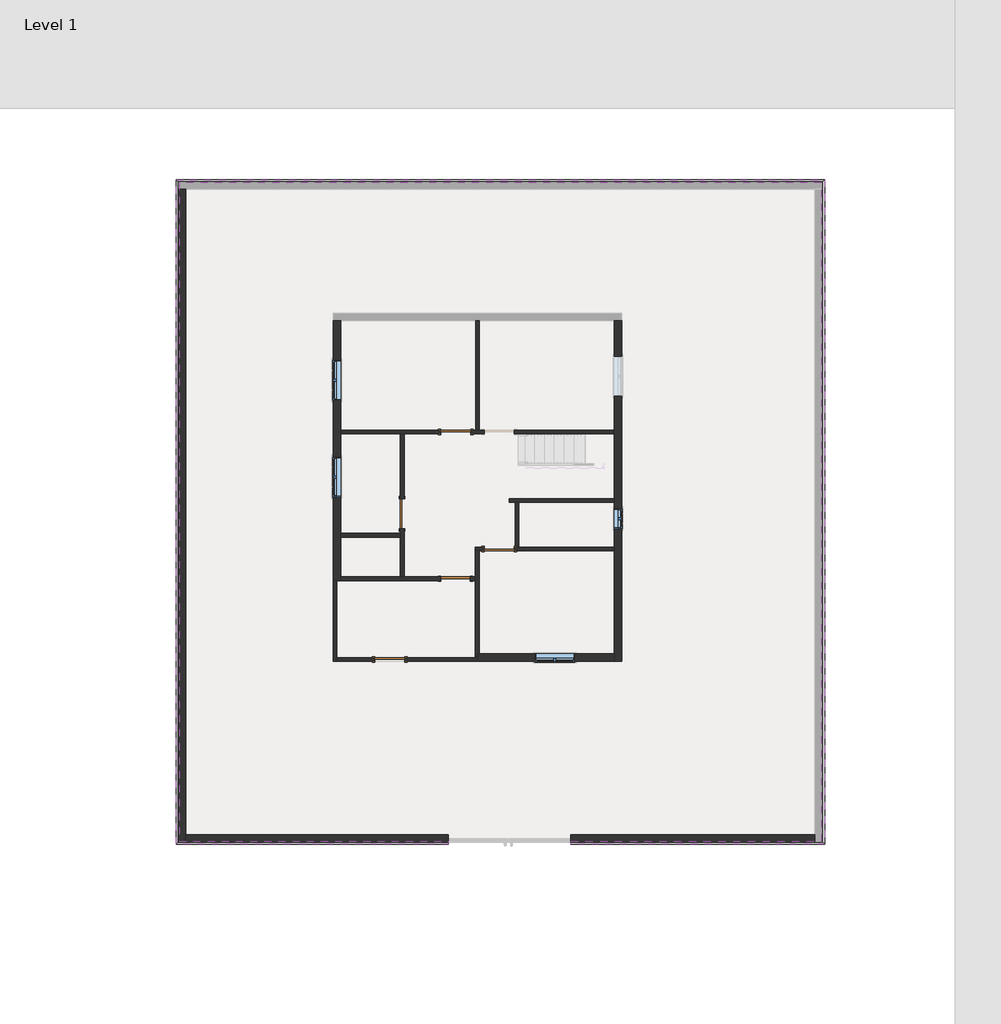
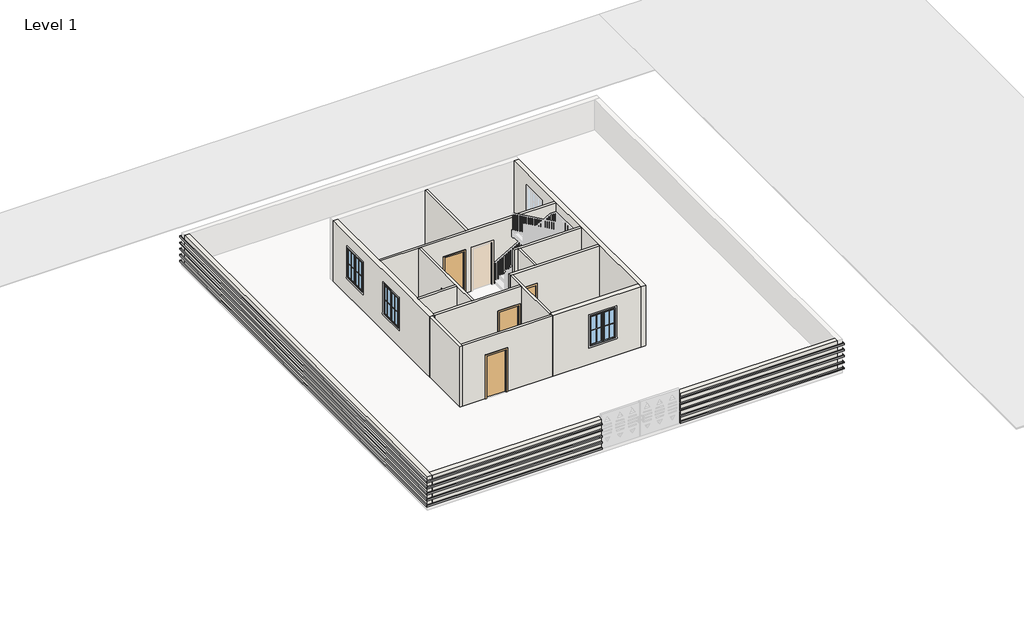
# One storey, part 1 of 3: 17 walls, 5 doors, 5 proxies, 4 windows.
"""IFC4 building model written with IfcOpenShell, lengths in millimetres."""

from ifc_helpers import new_model, si_unit, frame, origin, origin_with_axes, place, context, project, spatial, polyline, outline, extrude, faceted_brep, transform, mapped, element, save
from components import door_305aa2a5, door_e5f9f3c4, window_c417fced, window_8377141f

model = new_model("IFC4")

# Units and contexts
model_context = context("Model", 3, world=origin())
ifc_project = project(units=[si_unit("LENGTHUNIT", "METRE", prefix="MILLI")], contexts=[model_context])

# Site, building, storey
site = spatial("IfcSite", under=ifc_project)
building = spatial("IfcBuilding", under=site)
storey = spatial("IfcBuildingStorey", under=building, Name="Level 1", Elevation=0.0)

# Proxies
placement = place(None, origin())
element("IfcBuildingElementProxy", 1, Name="Reveal", ObjectType="Reveal", at=placement, inside=storey, context=model_context, shape_type="SweptSolid", body=[
    extrude(outline(polyline([(6441.1741, -3294.1944476), (6441.1741, -3386.2694476), (-1901.6163616, -3386.2694476), (-1809.5413616, -3294.1944476), (6441.1741, -3294.1944476)])), frame((0.0, 0.0, 50.8), z_axis=(0.0, 0.0, 1.0), x_axis=(1.0, 0.0, 0.0)), (0.0, 0.0, 1.0), 67.7333333),
    extrude(outline(polyline([(17875.4586384, -3294.270749), (17967.5336384, -3386.345749), (10185.6086384, -3386.345749), (10185.6086384, -3294.270749), (17875.4586384, -3294.270749)])), frame((0.0, 0.0, 50.8), z_axis=(0.0, 0.0, 1.0), x_axis=(1.0, 0.0, 0.0)), (0.0, 0.0, 1.0), 67.7333333),
    extrude(outline(polyline([(17875.4586384, 16898.729251), (17967.5336384, 16990.804251), (17967.5336384, -3386.345749), (17875.4586384, -3294.270749), (17875.4586384, 16898.729251)])), frame((0.0, 0.0, 50.8), z_axis=(0.0, 0.0, 1.0), x_axis=(1.0, 0.0, 0.0)), (0.0, 0.0, 1.0), 67.7333333),
    extrude(outline(polyline([(-1809.5413616, 16898.729251), (-1901.6163616, 16990.804251), (17967.5336384, 16990.804251), (17875.4586384, 16898.729251), (-1809.5413616, 16898.729251)])), frame((0.0, 0.0, 50.8), z_axis=(0.0, 0.0, 1.0), x_axis=(1.0, 0.0, 0.0)), (0.0, 0.0, 1.0), 67.7333333),
    extrude(outline(polyline([(-1809.5413616, -3294.1944476), (-1901.6163616, -3386.2694476), (-1901.6163616, 16990.804251), (-1809.5413616, 16898.729251), (-1809.5413616, -3294.1944476)])), frame((0.0, 0.0, 50.8), z_axis=(0.0, 0.0, 1.0), x_axis=(1.0, 0.0, 0.0)), (0.0, 0.0, 1.0), 67.7333333),
])
element("IfcBuildingElementProxy", 2, Name="Reveal", ObjectType="Reveal", at=placement, inside=storey, context=model_context, shape_type="SweptSolid", body=[
    extrude(outline(polyline([(6441.1741, -3294.1944476), (6441.1741, -3386.2694476), (-1901.6163616, -3386.2694476), (-1809.5413616, -3294.1944476), (6441.1741, -3294.1944476)])), frame((0.0, 0.0, 355.6), z_axis=(0.0, 0.0, 1.0), x_axis=(1.0, 0.0, 0.0)), (0.0, 0.0, 1.0), 67.7333333),
    extrude(outline(polyline([(17875.4586384, -3294.270749), (17967.5336384, -3386.345749), (10185.6086384, -3386.345749), (10185.6086384, -3294.270749), (17875.4586384, -3294.270749)])), frame((0.0, 0.0, 355.6), z_axis=(0.0, 0.0, 1.0), x_axis=(1.0, 0.0, 0.0)), (0.0, 0.0, 1.0), 67.7333333),
    extrude(outline(polyline([(17875.4586384, 16898.729251), (17967.5336384, 16990.804251), (17967.5336384, -3386.345749), (17875.4586384, -3294.270749), (17875.4586384, 16898.729251)])), frame((0.0, 0.0, 355.6), z_axis=(0.0, 0.0, 1.0), x_axis=(1.0, 0.0, 0.0)), (0.0, 0.0, 1.0), 67.7333333),
    extrude(outline(polyline([(-1809.5413616, 16898.729251), (-1901.6163616, 16990.804251), (17967.5336384, 16990.804251), (17875.4586384, 16898.729251), (-1809.5413616, 16898.729251)])), frame((0.0, 0.0, 355.6), z_axis=(0.0, 0.0, 1.0), x_axis=(1.0, 0.0, 0.0)), (0.0, 0.0, 1.0), 67.7333333),
    extrude(outline(polyline([(-1809.5413616, -3294.1944476), (-1901.6163616, -3386.2694476), (-1901.6163616, 16990.804251), (-1809.5413616, 16898.729251), (-1809.5413616, -3294.1944476)])), frame((0.0, 0.0, 355.6), z_axis=(0.0, 0.0, 1.0), x_axis=(1.0, 0.0, 0.0)), (0.0, 0.0, 1.0), 67.7333333),
])
element("IfcBuildingElementProxy", 3, Name="Reveal", ObjectType="Reveal", at=placement, inside=storey, context=model_context, shape_type="SweptSolid", body=[
    extrude(outline(polyline([(6441.1741, -3294.1944476), (6441.1741, -3386.2694476), (-1901.6163616, -3386.2694476), (-1809.5413616, -3294.1944476), (6441.1741, -3294.1944476)])), frame((0.0, 0.0, 660.4), z_axis=(0.0, 0.0, 1.0), x_axis=(1.0, 0.0, 0.0)), (0.0, 0.0, 1.0), 67.7333333),
    extrude(outline(polyline([(17875.4586384, -3294.270749), (17967.5336384, -3386.345749), (10185.6086384, -3386.345749), (10185.6086384, -3294.270749), (17875.4586384, -3294.270749)])), frame((0.0, 0.0, 660.4), z_axis=(0.0, 0.0, 1.0), x_axis=(1.0, 0.0, 0.0)), (0.0, 0.0, 1.0), 67.7333333),
    extrude(outline(polyline([(17875.4586384, 16898.729251), (17967.5336384, 16990.804251), (17967.5336384, -3386.345749), (17875.4586384, -3294.270749), (17875.4586384, 16898.729251)])), frame((0.0, 0.0, 660.4), z_axis=(0.0, 0.0, 1.0), x_axis=(1.0, 0.0, 0.0)), (0.0, 0.0, 1.0), 67.7333333),
    extrude(outline(polyline([(-1809.5413616, 16898.729251), (-1901.6163616, 16990.804251), (17967.5336384, 16990.804251), (17875.4586384, 16898.729251), (-1809.5413616, 16898.729251)])), frame((0.0, 0.0, 660.4), z_axis=(0.0, 0.0, 1.0), x_axis=(1.0, 0.0, 0.0)), (0.0, 0.0, 1.0), 67.7333333),
    extrude(outline(polyline([(-1809.5413616, -3294.1944476), (-1901.6163616, -3386.2694476), (-1901.6163616, 16990.804251), (-1809.5413616, 16898.729251), (-1809.5413616, -3294.1944476)])), frame((0.0, 0.0, 660.4), z_axis=(0.0, 0.0, 1.0), x_axis=(1.0, 0.0, 0.0)), (0.0, 0.0, 1.0), 67.7333333),
])
element("IfcBuildingElementProxy", 4, Name="Reveal", ObjectType="Reveal", at=placement, inside=storey, context=model_context, shape_type="SweptSolid", body=[
    extrude(outline(polyline([(6441.1741, -3294.1944476), (6441.1741, -3386.2694476), (-1901.6163616, -3386.2694476), (-1809.5413616, -3294.1944476), (6441.1741, -3294.1944476)])), frame((0.0, 0.0, 965.2), z_axis=(0.0, 0.0, 1.0), x_axis=(1.0, 0.0, 0.0)), (0.0, 0.0, 1.0), 67.7333333),
    extrude(outline(polyline([(17875.4586384, -3294.270749), (17967.5336384, -3386.345749), (10185.6086384, -3386.345749), (10185.6086384, -3294.270749), (17875.4586384, -3294.270749)])), frame((0.0, 0.0, 965.2), z_axis=(0.0, 0.0, 1.0), x_axis=(1.0, 0.0, 0.0)), (0.0, 0.0, 1.0), 67.7333333),
    extrude(outline(polyline([(17875.4586384, 16898.729251), (17967.5336384, 16990.804251), (17967.5336384, -3386.345749), (17875.4586384, -3294.270749), (17875.4586384, 16898.729251)])), frame((0.0, 0.0, 965.2), z_axis=(0.0, 0.0, 1.0), x_axis=(1.0, 0.0, 0.0)), (0.0, 0.0, 1.0), 67.7333333),
    extrude(outline(polyline([(-1809.5413616, 16898.729251), (-1901.6163616, 16990.804251), (17967.5336384, 16990.804251), (17875.4586384, 16898.729251), (-1809.5413616, 16898.729251)])), frame((0.0, 0.0, 965.2), z_axis=(0.0, 0.0, 1.0), x_axis=(1.0, 0.0, 0.0)), (0.0, 0.0, 1.0), 67.7333333),
    extrude(outline(polyline([(-1809.5413616, -3294.1944476), (-1901.6163616, -3386.2694476), (-1901.6163616, 16990.804251), (-1809.5413616, 16898.729251), (-1809.5413616, -3294.1944476)])), frame((0.0, 0.0, 965.2), z_axis=(0.0, 0.0, 1.0), x_axis=(1.0, 0.0, 0.0)), (0.0, 0.0, 1.0), 67.7333333),
])
element("IfcBuildingElementProxy", 5, Name="Reveal", ObjectType="Reveal", at=placement, inside=storey, context=model_context, shape_type="SweptSolid", body=[
    extrude(outline(polyline([(6441.1741, -3294.1944476), (6441.1741, -3386.2694476), (-1901.6163616, -3386.2694476), (-1809.5413616, -3294.1944476), (6441.1741, -3294.1944476)])), frame((0.0, 0.0, 1270.0), z_axis=(0.0, 0.0, 1.0), x_axis=(1.0, 0.0, 0.0)), (0.0, 0.0, 1.0), 67.7333333),
    extrude(outline(polyline([(17875.4586384, -3294.270749), (17967.5336384, -3386.345749), (10185.6086384, -3386.345749), (10185.6086384, -3294.270749), (17875.4586384, -3294.270749)])), frame((0.0, 0.0, 1270.0), z_axis=(0.0, 0.0, 1.0), x_axis=(1.0, 0.0, 0.0)), (0.0, 0.0, 1.0), 67.7333333),
    extrude(outline(polyline([(17875.4586384, 16898.729251), (17967.5336384, 16990.804251), (17967.5336384, -3386.345749), (17875.4586384, -3294.270749), (17875.4586384, 16898.729251)])), frame((0.0, 0.0, 1270.0), z_axis=(0.0, 0.0, 1.0), x_axis=(1.0, 0.0, 0.0)), (0.0, 0.0, 1.0), 67.7333333),
    extrude(outline(polyline([(-1809.5413616, 16898.729251), (-1901.6163616, 16990.804251), (17967.5336384, 16990.804251), (17875.4586384, 16898.729251), (-1809.5413616, 16898.729251)])), frame((0.0, 0.0, 1270.0), z_axis=(0.0, 0.0, 1.0), x_axis=(1.0, 0.0, 0.0)), (0.0, 0.0, 1.0), 67.7333333),
    extrude(outline(polyline([(-1809.5413616, -3294.1944476), (-1901.6163616, -3386.2694476), (-1901.6163616, 16990.804251), (-1809.5413616, 16898.729251), (-1809.5413616, -3294.1944476)])), frame((0.0, 0.0, 1270.0), z_axis=(0.0, 0.0, 1.0), x_axis=(1.0, 0.0, 0.0)), (0.0, 0.0, 1.0), 67.7333333),
])

# Doors
door_shape = door_305aa2a5(model_context)
element("IfcDoor", 6, ObjectType="Single-Flush : 36\" x 84\"", at=placement, inside=storey, context=model_context, shape_type="MappedRepresentation", body=[
    mapped(door_shape, transform((5022.9818578, 6750.05, 0.0), x_axis=(0.0, -1.0, 0.0), y_axis=(1.0, 0.0, 0.0), z_axis=(0.0, 0.0, 1.0))),
])
door_2_shape = door_e5f9f3c4(model_context)
element("IfcDoor", 7, ObjectType="Single-Flush : 36\" x 84\"", at=placement, inside=storey, context=model_context, shape_type="MappedRepresentation", body=[
    mapped(door_2_shape, transform((6667.5, 9251.95, 0.0), x_axis=(1.0, 0.0, 0.0), y_axis=(0.0, 1.0, 0.0), z_axis=(0.0, 0.0, 1.0))),
])
element("IfcDoor", 8, ObjectType="Single-Flush : 36\" x 84\"", at=placement, inside=storey, context=model_context, shape_type="MappedRepresentation", body=[
    mapped(door_2_shape, transform((8001.0, 5670.55, 0.0), x_axis=(-1.0, 0.0, 0.0), y_axis=(0.0, -1.0, 0.0), z_axis=(0.0, 0.0, 1.0))),
])
element("IfcDoor", 9, ObjectType="Single-Flush : 36\" x 84\"", at=placement, inside=storey, context=model_context, shape_type="MappedRepresentation", body=[
    mapped(door_2_shape, transform((6658.76875, 4756.15, 0.0), x_axis=(1.0, 0.0, 0.0), y_axis=(0.0, 1.0, 0.0), z_axis=(0.0, 0.0, 1.0))),
])
element("IfcDoor", 10, ObjectType="Single-Flush : 36\" x 84\"", at=placement, inside=storey, context=model_context, shape_type="MappedRepresentation", body=[
    mapped(door_2_shape, transform((4641.85, 2279.65, 0.0), x_axis=(1.0, 0.0, 0.0), y_axis=(0.0, 1.0, 0.0), z_axis=(0.0, 0.0, 1.0))),
])

# Walls
element("IfcWall", 11, ObjectType="Generic - 5\"", at=placement, inside=storey, context=model_context, shape_type="Brep", body=[
    faceted_brep([(7115.96875, 4699.0, 2133.6), (7115.96875, 4699.0, 0.0), (7264.4, 4699.0, 0.0), (7264.4, 4699.0, 3048.0), (3136.9, 4699.0, 3048.0), (3136.9, 4699.0, 0.0), (6201.56875, 4699.0, 0.0), (6201.56875, 4699.0, 2133.6), (7264.4, 4813.3, 0.0), (7115.96875, 4813.3, 0.0), (7115.96875, 4813.3, 2133.6), (6201.56875, 4813.3, 2133.6), (6201.56875, 4813.3, 0.0), (5080.1318578, 4813.3, 0.0), (4965.8318578, 4813.3, 0.0), (3136.9, 4813.3, 0.0), (3136.9, 4813.3, 3048.0), (4965.8318578, 4813.3, 3048.0), (5080.1318578, 4813.3, 3048.0), (7264.4, 4813.3, 3048.0)], [[[0, 1, 2, 3, 4, 5, 6, 7]], [[8, 9, 10, 11, 12, 13, 14, 15, 16, 17, 18, 19]], [[6, 5, 15, 14, 13, 12]], [[2, 1, 9, 8]], [[4, 3, 19, 18, 17, 16]], [[5, 4, 16, 15]], [[3, 2, 8, 19]], [[10, 9, 1, 0]], [[11, 10, 0, 7]], [[12, 11, 7, 6]]]),
])
element("IfcWall", 12, ObjectType="Generic - 5\"", at=placement, inside=storey, context=model_context, shape_type="SweptSolid", body=[
    extrude(outline(polyline([(4965.8318578, 6032.5), (3136.9, 6032.5), (3136.9, 6146.8), (4965.8318578, 6146.8), (4965.8318578, 6032.5)])), origin_with_axes(), (0.0, 0.0, 1.0), 3048.0),
])
element("IfcWall", 13, ObjectType="Generic - 5\"", at=placement, inside=storey, context=model_context, shape_type="Brep", body=[
    faceted_brep([(5080.1318578, 4813.3, 0.0), (5080.1318578, 6292.85, 0.0), (5080.1318578, 6292.85, 2133.6), (5080.1318578, 7207.25, 2133.6), (5080.1318578, 7207.25, 0.0), (5080.1318578, 9182.1, 0.0), (5080.1318578, 9182.1, 3048.0), (5080.1318578, 4813.3, 3048.0), (4965.8318578, 6292.85, 2133.6), (4965.8318578, 6292.85, 0.0), (4965.8318578, 6146.8, 0.0), (4965.8318578, 6032.5, 0.0), (4965.8318578, 4813.3, 0.0), (4965.8318578, 4813.3, 3048.0), (4965.8318578, 6032.5, 3048.0), (4965.8318578, 6146.8, 3048.0), (4965.8318578, 9182.1, 3048.0), (4965.8318578, 9182.1, 0.0), (4965.8318578, 7207.25, 0.0), (4965.8318578, 7207.25, 2133.6)], [[[0, 1, 2, 3, 4, 5, 6, 7]], [[8, 9, 10, 11, 12, 13, 14, 15, 16, 17, 18, 19]], [[18, 17, 5, 4]], [[12, 11, 10, 9, 1, 0]], [[6, 5, 17, 16]], [[7, 6, 16, 15, 14, 13]], [[0, 7, 13, 12]], [[2, 1, 9, 8]], [[3, 2, 8, 19]], [[4, 3, 19, 18]]]),
])
element("IfcWall", 14, ObjectType="Generic - 5\"", at=placement, inside=storey, context=model_context, shape_type="Brep", body=[
    faceted_brep([(7124.7, 9194.8, 2133.6), (7124.7, 9194.8, 0.0), (7543.8, 9194.8, 0.0), (7543.8, 9194.8, 2133.6), (8458.2, 9194.8, 2133.6), (8458.2, 9194.8, 0.0), (11518.9, 9194.8, 0.0), (11518.9, 9194.8, 3048.0), (3136.9, 9194.8, 3048.0), (3136.9, 9194.8, 0.0), (6210.3, 9194.8, 0.0), (6210.3, 9194.8, 2133.6), (7543.8, 9309.1, 0.0), (7391.4, 9309.1, 0.0), (7277.1, 9309.1, 0.0), (7124.7, 9309.1, 0.0), (7124.7, 9309.1, 2133.6), (6210.3, 9309.1, 2133.6), (6210.3, 9309.1, 0.0), (3136.9, 9309.1, 0.0), (3136.9, 9309.1, 3048.0), (7277.1, 9309.1, 3048.0), (7391.4, 9309.1, 3048.0), (11518.9, 9309.1, 3048.0), (11518.9, 9309.1, 0.0), (8458.2, 9309.1, 0.0), (8458.2, 9309.1, 2133.6), (7543.8, 9309.1, 2133.6)], [[[0, 1, 2, 3, 4, 5, 6, 7, 8, 9, 10, 11]], [[12, 13, 14, 15, 16, 17, 18, 19, 20, 21, 22, 23, 24, 25, 26, 27]], [[25, 24, 6, 5]], [[10, 9, 19, 18]], [[2, 1, 15, 14, 13, 12]], [[8, 7, 23, 22, 21, 20]], [[7, 6, 24, 23]], [[9, 8, 20, 19]], [[3, 2, 12, 27]], [[4, 3, 27, 26]], [[5, 4, 26, 25]], [[16, 15, 1, 0]], [[17, 16, 0, 11]], [[18, 17, 11, 10]]]),
])
element("IfcWall", 15, ObjectType="Generic - 5\"", at=placement, inside=storey, context=model_context, shape_type="SweptSolid", body=[
    extrude(outline(polyline([(7277.1, 9309.1), (7277.1, 12661.9), (7391.4, 12661.9), (7391.4, 9309.1), (7277.1, 9309.1)])), origin_with_axes(), (0.0, 0.0, 1.0), 3048.0),
])
element("IfcWall", 16, ObjectType="Generic - 5\"", at=placement, inside=storey, context=model_context, shape_type="Brep", body=[
    faceted_brep([(2908.3, 4699.0, 0.0), (2908.3, 2222.5, 0.0), (2908.3, 2222.5, 3048.0), (2908.3, 4699.0, 3048.0), (3022.6, 4699.0, 0.0), (3022.6, 4699.0, 3048.0), (3022.6, 2336.8, 3048.0), (3022.6, 2222.5, 3048.0), (3022.6, 2222.5, 0.0), (3022.6, 2336.8, 0.0)], [[[0, 1, 2, 3]], [[4, 5, 6, 7, 8, 9]], [[1, 0, 4, 9, 8]], [[3, 2, 7, 6, 5]], [[0, 3, 5, 4]], [[2, 1, 8, 7]]]),
])
element("IfcWall", 17, ObjectType="Generic - 5\"", at=placement, inside=storey, context=model_context, shape_type="Brep", body=[
    faceted_brep([(5099.05, 2222.5, 2133.6), (5099.05, 2222.5, 0.0), (7321.55, 2222.5, 0.0), (7321.55, 2222.5, 3048.0), (3022.6, 2222.5, 3048.0), (3022.6, 2222.5, 0.0), (4184.65, 2222.5, 0.0), (4184.65, 2222.5, 2133.6), (7321.55, 2336.8, 0.0), (7264.4, 2336.8, 0.0), (5099.05, 2336.8, 0.0), (5099.05, 2336.8, 2133.6), (4184.65, 2336.8, 2133.6), (4184.65, 2336.8, 0.0), (3022.6, 2336.8, 0.0), (3022.6, 2336.8, 3048.0), (7264.4, 2336.8, 3048.0), (7321.55, 2336.8, 3048.0)], [[[0, 1, 2, 3, 4, 5, 6, 7]], [[8, 9, 10, 11, 12, 13, 14, 15, 16, 17]], [[6, 5, 14, 13]], [[2, 1, 10, 9, 8]], [[3, 2, 8, 17]], [[4, 3, 17, 16, 15]], [[5, 4, 15, 14]], [[11, 10, 1, 0]], [[12, 11, 0, 7]], [[13, 12, 7, 6]]]),
])
element("IfcWall", 18, ObjectType="Generic - 5\"", at=placement, inside=storey, context=model_context, shape_type="Brep", body=[
    faceted_brep([(11518.9, 7213.6, 0.0), (8305.8, 7213.6, 0.0), (8305.8, 7213.6, 3048.0), (11518.9, 7213.6, 3048.0), (11518.9, 7099.3, 0.0), (11518.9, 7099.3, 3048.0), (8597.9, 7099.3, 3048.0), (8483.6, 7099.3, 3048.0), (8305.8, 7099.3, 3048.0), (8305.8, 7099.3, 0.0), (8483.6, 7099.3, 0.0), (8597.9, 7099.3, 0.0)], [[[0, 1, 2, 3]], [[4, 5, 6, 7, 8, 9, 10, 11]], [[1, 0, 4, 11, 10, 9]], [[2, 1, 9, 8]], [[3, 2, 8, 7, 6, 5]], [[0, 3, 5, 4]]]),
])
element("IfcWall", 19, ObjectType="Generic - 5\"", at=placement, inside=storey, context=model_context, shape_type="SweptSolid", body=[
    extrude(outline(polyline([(8483.6, 5727.7), (8483.6, 7099.3), (8597.9, 7099.3), (8597.9, 5727.7), (8483.6, 5727.7)])), origin_with_axes(), (0.0, 0.0, 1.0), 3048.0),
])
element("IfcWall", 20, ObjectType="Generic - 5\"", at=placement, inside=storey, context=model_context, shape_type="Brep", body=[
    faceted_brep([(7543.8, 5727.7, 2133.6), (7543.8, 5727.7, 0.0), (7264.4, 5727.7, 0.0), (7264.4, 5727.7, 3048.0), (8483.6, 5727.7, 3048.0), (8597.9, 5727.7, 3048.0), (11518.9, 5727.7, 3048.0), (11518.9, 5727.7, 0.0), (8597.9, 5727.7, 0.0), (8483.6, 5727.7, 0.0), (8458.2, 5727.7, 0.0), (8458.2, 5727.7, 2133.6), (7264.4, 5613.4, 0.0), (7378.7, 5613.4, 0.0), (7543.8, 5613.4, 0.0), (7543.8, 5613.4, 2133.6), (8458.2, 5613.4, 2133.6), (8458.2, 5613.4, 0.0), (11518.9, 5613.4, 0.0), (11518.9, 5613.4, 3048.0), (7378.7, 5613.4, 3048.0), (7264.4, 5613.4, 3048.0)], [[[0, 1, 2, 3, 4, 5, 6, 7, 8, 9, 10, 11]], [[12, 13, 14, 15, 16, 17, 18, 19, 20, 21]], [[2, 1, 14, 13, 12]], [[10, 9, 8, 7, 18, 17]], [[6, 5, 4, 3, 21, 20, 19]], [[7, 6, 19, 18]], [[3, 2, 12, 21]], [[15, 14, 1, 0]], [[16, 15, 0, 11]], [[17, 16, 11, 10]]]),
])
element("IfcWall", 21, ObjectType="Generic - 5\"", at=placement, inside=storey, context=model_context, shape_type="Brep", body=[
    faceted_brep([(7264.4, 5613.4, 0.0), (7264.4, 4813.3, 0.0), (7264.4, 4699.0, 0.0), (7264.4, 2336.8, 0.0), (7264.4, 2336.8, 3048.0), (7264.4, 4699.0, 3048.0), (7264.4, 4813.3, 3048.0), (7264.4, 5613.4, 3048.0), (7378.7, 5613.4, 0.0), (7378.7, 5613.4, 3048.0), (7378.7, 2451.1, 3048.0), (7378.7, 2451.1, 0.0), (7321.55, 2451.1, 0.0), (7321.55, 2336.8, 0.0), (7321.55, 2336.8, 3048.0), (7321.55, 2451.1, 3048.0)], [[[0, 1, 2, 3, 4, 5, 6, 7]], [[8, 9, 10, 11]], [[3, 2, 1, 0, 8, 11, 12, 13]], [[7, 6, 5, 4, 14, 15, 10, 9]], [[0, 7, 9, 8]], [[4, 3, 13, 14]], [[13, 12, 15, 14]], [[12, 11, 10, 15]]]),
])
element("IfcWall", 22, ObjectType="Generic - 8\"", at=placement, inside=storey, context=model_context, shape_type="Brep", body=[
    faceted_brep([(11518.9, 12661.9, 0.0), (11518.9, 9309.1, 0.0), (11518.9, 9194.8, 0.0), (11518.9, 7213.6, 0.0), (11518.9, 7099.3, 0.0), (11518.9, 5727.7, 0.0), (11518.9, 5613.4, 0.0), (11518.9, 2451.1, 0.0), (11518.9, 2222.5, 0.0), (11518.9, 2222.5, 3048.0), (11518.9, 2451.1, 3048.0), (11518.9, 5613.4, 3048.0), (11518.9, 5727.7, 3048.0), (11518.9, 7099.3, 3048.0), (11518.9, 7213.6, 3048.0), (11518.9, 9194.8, 3048.0), (11518.9, 9309.1, 3048.0), (11518.9, 12661.9, 3048.0), (11518.9, 10352.0875, 2438.4), (11518.9, 10352.0875, 914.4), (11518.9, 11571.2875, 914.4), (11518.9, 11571.2875, 2438.4), (11518.9, 6292.85, 1828.8), (11518.9, 6292.85, 914.4), (11518.9, 6902.45, 914.4), (11518.9, 6902.45, 1828.8), (11747.5, 12661.9, 0.0), (11747.5, 12661.9, 3048.0), (11747.5, 2222.5, 3048.0), (11747.5, 2222.5, 0.0), (11747.5, 10352.0875, 2438.4), (11747.5, 11571.2875, 2438.4), (11747.5, 11571.2875, 914.4), (11747.5, 10352.0875, 914.4), (11747.5, 6292.85, 1828.8), (11747.5, 6902.45, 1828.8), (11747.5, 6902.45, 914.4), (11747.5, 6292.85, 914.4)], [[[0, 1, 2, 3, 4, 5, 6, 7, 8, 9, 10, 11, 12, 13, 14, 15, 16, 17], [18, 19, 20, 21], [22, 23, 24, 25]], [[26, 27, 28, 29], [30, 31, 32, 33], [34, 35, 36, 37]], [[8, 7, 6, 5, 4, 3, 2, 1, 0, 26, 29]], [[0, 17, 27, 26]], [[9, 8, 29, 28]], [[19, 18, 30, 33]], [[20, 19, 33, 32]], [[21, 20, 32, 31]], [[18, 21, 31, 30]], [[23, 22, 34, 37]], [[24, 23, 37, 36]], [[25, 24, 36, 35]], [[22, 25, 35, 34]], [[17, 16, 15, 14, 13, 12, 11, 10, 9, 28, 27]]]),
])
element("IfcWall", 23, ObjectType="Generic - 8\"", at=placement, inside=storey, context=model_context, shape_type="Brep", body=[
    faceted_brep([(2908.3, 12661.9, 0.0), (2908.3, 4699.0, 0.0), (2908.3, 4699.0, 3048.0), (2908.3, 12661.9, 3048.0), (2908.3, 8480.425, 2438.4), (2908.3, 7261.225, 2438.4), (2908.3, 7261.225, 914.4), (2908.3, 8480.425, 914.4), (2908.3, 11449.05, 2438.4), (2908.3, 10229.85, 2438.4), (2908.3, 10229.85, 914.4), (2908.3, 11449.05, 914.4), (3136.9, 12661.9, 0.0), (3136.9, 12661.9, 3048.0), (3136.9, 9309.1, 3048.0), (3136.9, 9194.8, 3048.0), (3136.9, 6146.8, 3048.0), (3136.9, 6032.5, 3048.0), (3136.9, 4813.3, 3048.0), (3136.9, 4699.0, 3048.0), (3136.9, 4699.0, 0.0), (3136.9, 4813.3, 0.0), (3136.9, 6032.5, 0.0), (3136.9, 6146.8, 0.0), (3136.9, 9194.8, 0.0), (3136.9, 9309.1, 0.0), (3136.9, 8480.425, 2438.4), (3136.9, 8480.425, 914.4), (3136.9, 7261.225, 914.4), (3136.9, 7261.225, 2438.4), (3136.9, 11449.05, 2438.4), (3136.9, 11449.05, 914.4), (3136.9, 10229.85, 914.4), (3136.9, 10229.85, 2438.4), (3022.6, 4699.0, 0.0), (3022.6, 4699.0, 3048.0)], [[[0, 1, 2, 3], [4, 5, 6, 7], [8, 9, 10, 11]], [[12, 13, 14, 15, 16, 17, 18, 19, 20, 21, 22, 23, 24, 25], [26, 27, 28, 29], [30, 31, 32, 33]], [[1, 0, 12, 25, 24, 23, 22, 21, 20, 34]], [[0, 3, 13, 12]], [[2, 1, 34, 20, 19, 35]], [[27, 26, 4, 7]], [[28, 27, 7, 6]], [[29, 28, 6, 5]], [[26, 29, 5, 4]], [[31, 30, 8, 11]], [[32, 31, 11, 10]], [[33, 32, 10, 9]], [[30, 33, 9, 8]], [[3, 2, 35, 19, 18, 17, 16, 15, 14, 13]]]),
])
element("IfcWall", 24, ObjectType="Generic - 8\"", at=placement, inside=storey, context=model_context, shape_type="Brep", body=[
    faceted_brep([(7321.55, 2222.5, 0.0), (11518.9, 2222.5, 0.0), (11518.9, 2222.5, 3048.0), (7321.55, 2222.5, 3048.0), (9090.81875, 2222.5, 2438.4), (10310.01875, 2222.5, 2438.4), (10310.01875, 2222.5, 914.4), (9090.81875, 2222.5, 914.4), (7321.55, 2451.1, 0.0), (7321.55, 2451.1, 3048.0), (7378.7, 2451.1, 3048.0), (11518.9, 2451.1, 3048.0), (11518.9, 2451.1, 0.0), (7378.7, 2451.1, 0.0), (9090.81875, 2451.1, 2438.4), (9090.81875, 2451.1, 914.4), (10310.01875, 2451.1, 914.4), (10310.01875, 2451.1, 2438.4), (7321.55, 2336.8, 0.0), (7321.55, 2336.8, 3048.0)], [[[0, 1, 2, 3], [4, 5, 6, 7]], [[8, 9, 10, 11, 12, 13], [14, 15, 16, 17]], [[1, 0, 18, 8, 13, 12]], [[0, 3, 19, 9, 8, 18]], [[2, 1, 12, 11]], [[15, 14, 4, 7]], [[16, 15, 7, 6]], [[17, 16, 6, 5]], [[14, 17, 5, 4]], [[3, 2, 11, 10, 9, 19]]]),
])
element("IfcWall", 25, ObjectType="Generic - 8\"", at=placement, inside=storey, context=model_context, shape_type="SweptSolid", body=[
    extrude(outline(polyline([(-3091.070749, 1524.0), (-3091.070749, 0.0), (-3319.670749, 0.0), (-3319.670749, 50.8), (-3294.270749, 50.8), (-3294.270749, 118.5333333), (-3319.670749, 118.5333333), (-3319.670749, 355.6), (-3294.270749, 355.6), (-3294.270749, 423.3333333), (-3319.670749, 423.3333333), (-3319.670749, 660.4), (-3294.270749, 660.4), (-3294.270749, 728.1333333), (-3319.670749, 728.1333333), (-3319.670749, 965.2), (-3294.270749, 965.2), (-3294.270749, 1032.9333333), (-3319.670749, 1032.9333333), (-3319.670749, 1270.0), (-3294.270749, 1270.0), (-3294.270749, 1337.7333333), (-3319.670749, 1337.7333333), (-3319.670749, 1524.0), (-3091.070749, 1524.0)])), frame((10185.6086384, 0.0, 0.0), z_axis=(1.0, 0.0, 0.0), x_axis=(0.0, 1.0, 0.0)), (0.0, 0.0, 1.0), 7486.65),
])
element("IfcWall", 26, ObjectType="Generic - 8\"", at=placement, inside=storey, context=model_context, shape_type="Brep", body=[
    faceted_brep([(-1606.3413616, -3319.5944476, 0.0), (-1606.3413616, -3090.9944476, 0.0), (-1606.3413616, 16695.529251, 0.0), (-1606.3413616, 16695.529251, 1524.0), (-1606.3413616, -3090.9944476, 1524.0), (-1606.3413616, -3319.5944476, 1524.0), (-1606.3413616, -3319.5944476, 1337.7333333), (-1606.3413616, -3294.1944476, 1337.7333333), (-1606.3413616, -3294.1944476, 1270.0), (-1606.3413616, -3319.5944476, 1270.0), (-1606.3413616, -3319.5944476, 1032.9333333), (-1606.3413616, -3294.1944476, 1032.9333333), (-1606.3413616, -3294.1944476, 965.2), (-1606.3413616, -3319.5944476, 965.2), (-1606.3413616, -3319.5944476, 728.1333333), (-1606.3413616, -3294.1944476, 728.1333333), (-1606.3413616, -3294.1944476, 660.4), (-1606.3413616, -3319.5944476, 660.4), (-1606.3413616, -3319.5944476, 423.3333333), (-1606.3413616, -3294.1944476, 423.3333333), (-1606.3413616, -3294.1944476, 355.6), (-1606.3413616, -3319.5944476, 355.6), (-1606.3413616, -3319.5944476, 118.5333333), (-1606.3413616, -3294.1944476, 118.5333333), (-1606.3413616, -3294.1944476, 50.8), (-1606.3413616, -3319.5944476, 50.8), (-1834.9413616, 16695.529251, 0.0), (-1834.9413616, -3319.5944476, 0.0), (-1834.9413616, -3319.5944476, 50.8), (-1834.9413616, 16695.529251, 50.8), (-1834.9413616, -3319.5944476, 1524.0), (-1834.9413616, 16695.529251, 1524.0), (-1834.9413616, 16695.529251, 1337.7333333), (-1834.9413616, -3319.5944476, 1337.7333333), (-1834.9413616, 16695.529251, 118.5333333), (-1834.9413616, -3319.5944476, 118.5333333), (-1834.9413616, -3319.5944476, 355.6), (-1834.9413616, 16695.529251, 355.6), (-1834.9413616, 16695.529251, 423.3333333), (-1834.9413616, -3319.5944476, 423.3333333), (-1834.9413616, -3319.5944476, 660.4), (-1834.9413616, 16695.529251, 660.4), (-1834.9413616, 16695.529251, 728.1333333), (-1834.9413616, -3319.5944476, 728.1333333), (-1834.9413616, -3319.5944476, 965.2), (-1834.9413616, 16695.529251, 965.2), (-1834.9413616, 16695.529251, 1032.9333333), (-1834.9413616, -3319.5944476, 1032.9333333), (-1834.9413616, -3319.5944476, 1270.0), (-1834.9413616, 16695.529251, 1270.0), (-1809.5413616, 16695.529251, 50.8), (-1809.5413616, 16695.529251, 118.5333333), (-1809.5413616, 16695.529251, 355.6), (-1809.5413616, 16695.529251, 423.3333333), (-1809.5413616, 16695.529251, 660.4), (-1809.5413616, 16695.529251, 728.1333333), (-1809.5413616, 16695.529251, 965.2), (-1809.5413616, 16695.529251, 1032.9333333), (-1809.5413616, 16695.529251, 1270.0), (-1809.5413616, 16695.529251, 1337.7333333), (-1809.5413616, -3294.1944476, 118.5333333), (-1809.5413616, -3294.1944476, 50.8), (-1809.5413616, -3294.1944476, 423.3333333), (-1809.5413616, -3294.1944476, 355.6), (-1809.5413616, -3294.1944476, 728.1333333), (-1809.5413616, -3294.1944476, 660.4), (-1809.5413616, -3294.1944476, 1032.9333333), (-1809.5413616, -3294.1944476, 965.2), (-1809.5413616, -3294.1944476, 1337.7333333), (-1809.5413616, -3294.1944476, 1270.0)], [[[0, 1, 2, 3, 4, 5, 6, 7, 8, 9, 10, 11, 12, 13, 14, 15, 16, 17, 18, 19, 20, 21, 22, 23, 24, 25]], [[26, 27, 28, 29]], [[30, 31, 32, 33]], [[34, 35, 36, 37]], [[38, 39, 40, 41]], [[42, 43, 44, 45]], [[46, 47, 48, 49]], [[2, 1, 0, 27, 26]], [[5, 4, 3, 31, 30]], [[3, 2, 26, 29, 50, 51, 34, 37, 52, 53, 38, 41, 54, 55, 42, 45, 56, 57, 46, 49, 58, 59, 32, 31]], [[5, 30, 33, 6]], [[27, 0, 25, 28]], [[35, 22, 21, 36]], [[39, 18, 17, 40]], [[43, 14, 13, 44]], [[47, 10, 9, 48]], [[51, 60, 23, 22, 35, 34]], [[24, 61, 50, 29, 28, 25]], [[60, 61, 24, 23]], [[61, 60, 51, 50]], [[53, 62, 19, 18, 39, 38]], [[20, 63, 52, 37, 36, 21]], [[62, 63, 20, 19]], [[63, 62, 53, 52]], [[55, 64, 15, 14, 43, 42]], [[16, 65, 54, 41, 40, 17]], [[64, 65, 16, 15]], [[65, 64, 55, 54]], [[57, 66, 11, 10, 47, 46]], [[12, 67, 56, 45, 44, 13]], [[66, 67, 12, 11]], [[67, 66, 57, 56]], [[59, 68, 7, 6, 33, 32]], [[8, 69, 58, 49, 48, 9]], [[68, 69, 8, 7]], [[69, 68, 59, 58]]]),
])
element("IfcWall", 27, ObjectType="Generic - 8\"", at=placement, inside=storey, context=model_context, shape_type="SweptSolid", body=[
    extrude(outline(polyline([(-3090.9944476, 1524.0), (-3090.9944476, 0.0), (-3319.5944476, 0.0), (-3319.5944476, 50.8), (-3294.1944476, 50.8), (-3294.1944476, 118.5333333), (-3319.5944476, 118.5333333), (-3319.5944476, 355.6), (-3294.1944476, 355.6), (-3294.1944476, 423.3333333), (-3319.5944476, 423.3333333), (-3319.5944476, 660.4), (-3294.1944476, 660.4), (-3294.1944476, 728.1333333), (-3319.5944476, 728.1333333), (-3319.5944476, 965.2), (-3294.1944476, 965.2), (-3294.1944476, 1032.9333333), (-3319.5944476, 1032.9333333), (-3319.5944476, 1270.0), (-3294.1944476, 1270.0), (-3294.1944476, 1337.7333333), (-3319.5944476, 1337.7333333), (-3319.5944476, 1524.0), (-3090.9944476, 1524.0)])), frame((-1606.3413616, 0.0, 0.0), z_axis=(1.0, 0.0, 0.0), x_axis=(0.0, 1.0, 0.0)), (0.0, 0.0, 1.0), 8047.5154616),
])

# Windows
window_shape = window_c417fced(model_context)
element("IfcWindow", 28, ObjectType="Window-Casement-Double : 24\" x 36\"", at=placement, inside=storey, context=model_context, shape_type="MappedRepresentation", body=[
    mapped(window_shape, transform((11633.2, 6597.65, 0.0), x_axis=(0.0, -1.0, 0.0), y_axis=(1.0, 0.0, 0.0), z_axis=(0.0, 0.0, 1.0))),
])
window_2_shape = window_8377141f(model_context)
element("IfcWindow", 29, ObjectType="Window-Casement-Double : 48\" x 60\"", at=placement, inside=storey, context=model_context, shape_type="MappedRepresentation", body=[
    mapped(window_2_shape, transform((9700.41875, 2336.8, 0.0), x_axis=(-1.0, 0.0, 0.0), y_axis=(0.0, -1.0, 0.0), z_axis=(0.0, 0.0, 1.0))),
])
element("IfcWindow", 30, ObjectType="Window-Casement-Double : 48\" x 60\"", at=placement, inside=storey, context=model_context, shape_type="MappedRepresentation", body=[
    mapped(window_2_shape, transform((3022.6, 7870.825, 0.0), x_axis=(0.0, 1.0, 0.0), y_axis=(-1.0, 0.0, 0.0), z_axis=(0.0, 0.0, 1.0))),
])
element("IfcWindow", 31, ObjectType="Window-Casement-Double : 48\" x 60\"", at=placement, inside=storey, context=model_context, shape_type="MappedRepresentation", body=[
    mapped(window_2_shape, transform((3022.6, 10839.45, 0.0), x_axis=(0.0, 1.0, 0.0), y_axis=(-1.0, 0.0, 0.0), z_axis=(0.0, 0.0, 1.0))),
])

save(model, "model.ifc")

# Revit data of these elements
# Type "Single-Flush : 36\" x 84\""
#   Type Mark = "1"
#   Construction Type Id = "MDOOR"
#   Assembly Code = "C1020"
#   Analytic Construction = "Metal"
#   Thickness = 0' - 2"
#   Heat Transfer Coefficient (U) = 0.651978 BTU/(h·ft²·°F)
#   Height = 7' - 0"
#   Trim Projection Ext = 0' - 1"
#   Trim Projection Int = 0' - 1"
#   Trim Width = 0' - 3"
#   Width = 3' - 0"
#   Define Thermal Properties by = 1
#   Define Thermal Properties by = 1
#   Door Material = Door - Panel
#   Frame Material = Door - Frame
#   Visual Light Transmittance = 0
#   Solar Heat Gain Coefficient = 0
#   Function = (empty or 0)
#   Wall Closure = (empty or 0)
# Type "Generic - 5\""
#   Assembly Code = "B2010"
#   Layers, outside or top first: 0' - 4 1/2" no material (function 1)
# Type "Generic - 8\""
#   Assembly Code = "B2010"
#   Layers, outside or top first: 0' - 9" "Parking Stripe" (function 1)
# Type "Window-Casement-Double : 24\" x 36\""
#   Type Mark = "14"
#   Fire Rating = "0.5h"
#   Assembly Code = "B2020100"
#   Analytic Construction = "Double glazing - domestic"
#   Frame Extension [instance default] = 0' - 0 1/4"
#   Window Inset [instance default] = 0' - 0"
#   Wall Thickness [instance default] = 0' - 6"
#   Interior Wall Closure [instance default] = 0' - 2 1/4"
#   Half Width = 1' - 0"
#   Visual Light Transmittance = 0.81
#   Thermal Resistance (R) = 1.8146 (h·ft²·°F)/BTU
#   Solar Heat Gain Coefficient = 0.76
#   Rough Width = 2' - 0 1/2"
#   Rough Height = 3' - 0 1/2"
#   Height = 3' - 0"
#   Heat Transfer Coefficient (U) = 0.5511 BTU/(h·ft²·°F)
#   Exterior Wall Closure [instance default] = 0' - 1 1/4"
#   Extension Jamb [instance default] = 0' - 2 1/4"
#   Default Sill Height = 3' - 0"
#   Width = 2' - 0"
#   Define Thermal Properties by = 0
#   Muntin Visibility = yes
#   Interior Trim Visibility [instance default] = yes
#   Exterior Trim Visibility [instance default] = yes
#   Extension Jamb Visibility [instance default] = yes
#   Interior Trim Material = Wood - Stained
#   Muntin Pattern = Muntin Pattern_2x2 : Muntin Pattern_2x2
#   Interior Trim = Trim-Window-Interior-Flat : Picture Frame
#   Interior Frame Material = Wood - Stained
#   Glass Panel Material = Glass
#   Exterior Trim Material = Clad - White
#   Exterior Trim = Trim-Window-Exterior-Flat : with Sill
#   Exterior Frame Material = Clad - White
#   Wall Closure = (empty or 0)
# Type "Window-Casement-Double : 48\" x 60\""
#   Type Mark = "17"
#   Fire Rating = "0.5h"
#   Assembly Code = "B2020100"
#   Analytic Construction = "Double glazing - domestic"
#   Frame Extension [instance default] = 0' - 0 1/4"
#   Window Inset [instance default] = 0' - 0"
#   Wall Thickness [instance default] = 0' - 6"
#   Interior Wall Closure [instance default] = 0' - 2 1/4"
#   Half Width = 2' - 0"
#   Visual Light Transmittance = 0.81
#   Thermal Resistance (R) = 1.8146 (h·ft²·°F)/BTU
#   Solar Heat Gain Coefficient = 0.76
#   Rough Width = 4' - 0 1/2"
#   Rough Height = 5' - 0 1/2"
#   Height = 5' - 0"
#   Heat Transfer Coefficient (U) = 0.5511 BTU/(h·ft²·°F)
#   Exterior Wall Closure [instance default] = 0' - 1 1/4"
#   Extension Jamb [instance default] = 0' - 2 1/4"
#   Default Sill Height = 3' - 0"
#   Width = 4' - 0"
#   Define Thermal Properties by = 0
#   Muntin Visibility = yes
#   Interior Trim Visibility [instance default] = yes
#   Exterior Trim Visibility [instance default] = yes
#   Extension Jamb Visibility [instance default] = yes
#   Interior Trim Material = Wood - Stained
#   Muntin Pattern = Muntin Pattern_2x2 : Muntin Pattern_2x2
#   Interior Trim = Trim-Window-Interior-Flat : Picture Frame
#   Interior Frame Material = Wood - Stained
#   Glass Panel Material = Glass
#   Exterior Trim Material = Clad - White
#   Exterior Trim = Trim-Window-Exterior-Flat : with Sill
#   Exterior Frame Material = Clad - White
#   Wall Closure = (empty or 0)
# Elements 6, 7, 8, 9, 10 (IfcDoor, "Single-Flush : 36\" x 84\"")
#   Phase Created = New Construction
#   Materials on its faces: "Door - Frame", "Door - Panel"
# Elements 11, 12, 13, 14, 15, 18, 19, 20, 21 (IfcWall, "Generic - 5\"")
#   Top Offset = 0' - 0"
#   Base Offset = 0' - 0"
#   wall height = 10' - 0"
#   Phase Created = New Construction
#   Base Constraint = Level 1
#   Top Constraint = Level 2
#   Materials on its faces: "Default Wall"
# Elements 16, 17 (IfcWall, "Generic - 5\"")
#   Top Offset = 0' - 0"
#   Base Offset = 0' - 0"
#   wall height = 10' - 0"
#   Phase Created = New Construction
#   Base Constraint = Level 1
#   Top Constraint = Level 2
#   Materials on its faces: "Default Wall", "Cherry"
# Elements 22, 24 (IfcWall, "Generic - 8\"")
#   Top Offset = 0' - 0"
#   Base Offset = 0' - 0"
#   Unconnected Height = 10' - 0"
#   wall height = 10' - 0"
#   Phase Created = New Construction
#   Base Constraint = Level 1
#   Materials on its faces: "Parking Stripe", "Cherry"
# Element 23 (IfcWall, "Generic - 8\"")
#   Top Offset = 0' - 0"
#   Base Offset = 0' - 0"
#   Unconnected Height = 10' - 0"
#   wall height = 10' - 0"
#   Phase Created = New Construction
#   Base Constraint = Level 1
#   Materials on its faces: "Parking Stripe", "Cherry", "Default Wall"
# Elements 25, 27 (IfcWall, "Generic - 8\"")
#   Top Offset = 0' - 0"
#   Base Offset = 0' - 0"
#   Unconnected Height = 5' - 0"
#   wall height = 5' - 0"
#   Phase Created = New Construction
#   Base Constraint = Level 1
#   Materials on its faces: "Parking Stripe", "Cherry", "Clad - White"
# Element 26 (IfcWall, "Generic - 8\"")
#   Top Offset = 0' - 0"
#   Base Offset = 0' - 0"
#   Unconnected Height = 5' - 0"
#   wall height = 5' - 0"
#   Phase Created = New Construction
#   Base Constraint = Level 1
#   Materials on its faces: "Parking Stripe", "Clad - White", "Cherry"
# Element 28 (IfcWindow, "Window-Casement-Double : 24\" x 36\"")
#   Mark = "5"
#   Window Inset = 0' - 0"
#   Interior Wall Closure = 0' - 2 1/4"
#   Frame Extension = 0' - 0 1/4"
#   Exterior Wall Closure = 0' - 1 1/4"
#   Interior Trim Visibility = yes
#   Exterior Trim Visibility = yes
#   Phase Created = New Construction
#   Materials on its faces: "Wood - Stained", "Glass", "Clad - White"
# Element 29 (IfcWindow, "Window-Casement-Double : 48\" x 60\"")
#   Mark = "1"
#   Window Inset = 0' - 0"
#   Interior Wall Closure = 0' - 2 1/4"
#   Frame Extension = 0' - 0 1/4"
#   Exterior Wall Closure = 0' - 1 1/4"
#   Interior Trim Visibility = yes
#   Exterior Trim Visibility = yes
#   Phase Created = New Construction
#   Materials on its faces: "Wood - Stained", "Glass", "Clad - White"
# Element 30 (IfcWindow, "Window-Casement-Double : 48\" x 60\"")
#   Mark = "2"
#   Window Inset = 0' - 0"
#   Interior Wall Closure = 0' - 2 1/4"
#   Frame Extension = 0' - 0 1/4"
#   Exterior Wall Closure = 0' - 1 1/4"
#   Interior Trim Visibility = yes
#   Exterior Trim Visibility = yes
#   Phase Created = New Construction
#   Materials on its faces: "Wood - Stained", "Glass", "Clad - White"
# Element 31 (IfcWindow, "Window-Casement-Double : 48\" x 60\"")
#   Mark = "3"
#   Window Inset = 0' - 0"
#   Interior Wall Closure = 0' - 2 1/4"
#   Frame Extension = 0' - 0 1/4"
#   Exterior Wall Closure = 0' - 1 1/4"
#   Interior Trim Visibility = yes
#   Exterior Trim Visibility = yes
#   Phase Created = New Construction
#   Materials on its faces: "Wood - Stained", "Glass", "Clad - White"
# Materials
#   "Door - Panel": class "Wood", colour RGB 210 159 95, transparency 0, Cost = 0
#   "Door - Frame": colour RGB 118 70 51, transparency 0, Cost = 0
#   "Parking Stripe": class "Paint", colour RGB 250 250 91, transparency 0, Cost = 0
#   "Wood - Stained": class "Wood", colour RGB 224 178 126, transparency 0, Cost = 0
#   "Glass": class "Glass", colour RGB 0 128 192, transparency 0.75, Description = "Soda Lime Glass", Cost = 0
#   "Clad - White": class "Wood", colour RGB 242 242 238, transparency 0, Cost = 0
#   "Default Wall": colour RGB 128 128 128, transparency 0, Cost = 0
#   "Cherry": class "Wood", colour RGB 226 177 128, transparency 0, Description = "Prunus Serotina", Cost = 0
